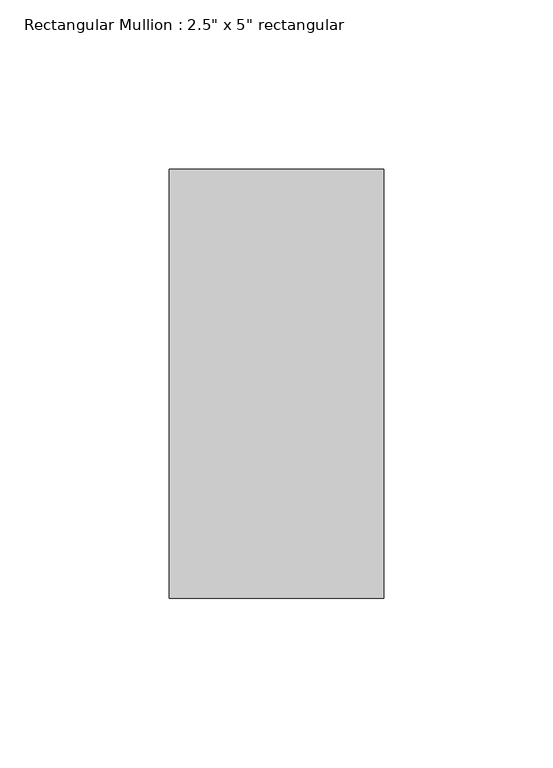
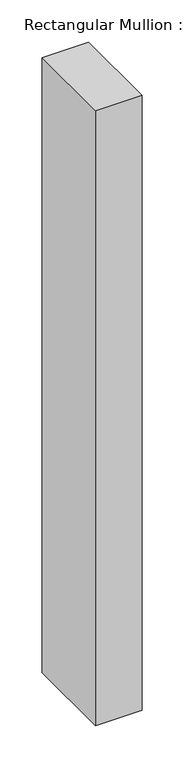
"""IFC4 building model written with IfcOpenShell, lengths in millimetres: member geometry."""

from ifc_helpers import new_model, si_unit, frame, origin, place, context, project, spatial, polyline, outline, extrude, source, transform, mapped, element, save


def member_a99653d8(model_context):
    return source(origin(), model_context, "Body", "SweptSolid", [
        extrude(outline(polyline([(31.75, 63.5), (31.75, -63.5), (-31.75, -63.5), (-31.75, 63.5), (31.75, 63.5)])), frame((0.0, 0.0, -889.8127727), z_axis=(0.0, 0.0, 1.0), x_axis=(1.0, 0.0, 0.0)), (0.0, 0.0, 1.0), 889.8127727),
    ])


if __name__ == "__main__":
    model = new_model("IFC4")
    model_context = context("Model", 3, world=origin())
    ifc_project = project(units=[si_unit("LENGTHUNIT", "METRE", prefix="MILLI")], contexts=[model_context])
    site = spatial("IfcSite", under=ifc_project)
    building = spatial("IfcBuilding", under=site)
    placement = place(None, origin())
    member_shape = member_a99653d8(model_context)
    element("IfcMember", 1, ObjectType="Rectangular Mullion : 2.5\" x 5\" rectangular", at=placement, inside=building, context=model_context, shape_type="MappedRepresentation", body=[
        mapped(member_shape, transform((0.0, 0.0, 0.0), x_axis=(1.0, 0.0, 0.0), y_axis=(0.0, 1.0, 0.0), z_axis=(0.0, 0.0, 1.0))),
    ])
    save(model, "model.ifc")

# Revit data of these elements
# Type "Rectangular Mullion : 2.5\" x 5\" rectangular"
#   built-in parameter 1007304 = 0.416667 (stored number, unit not read)
#   built-in parameter 1007301 = 0.104167 (stored number, unit not read)
#   built-in parameter 1007300 = 0.104167 (stored number, unit not read)
# Element 1 (IfcMember, "Rectangular Mullion : 2.5\" x 5\" rectangular")
#   Materials on its faces: "Aluminum"
# Materials
#   "Aluminum": class "Metal", colour RGB 247 247 247, transparency 0, Description = "Aluminum 6061", Cost = 0
